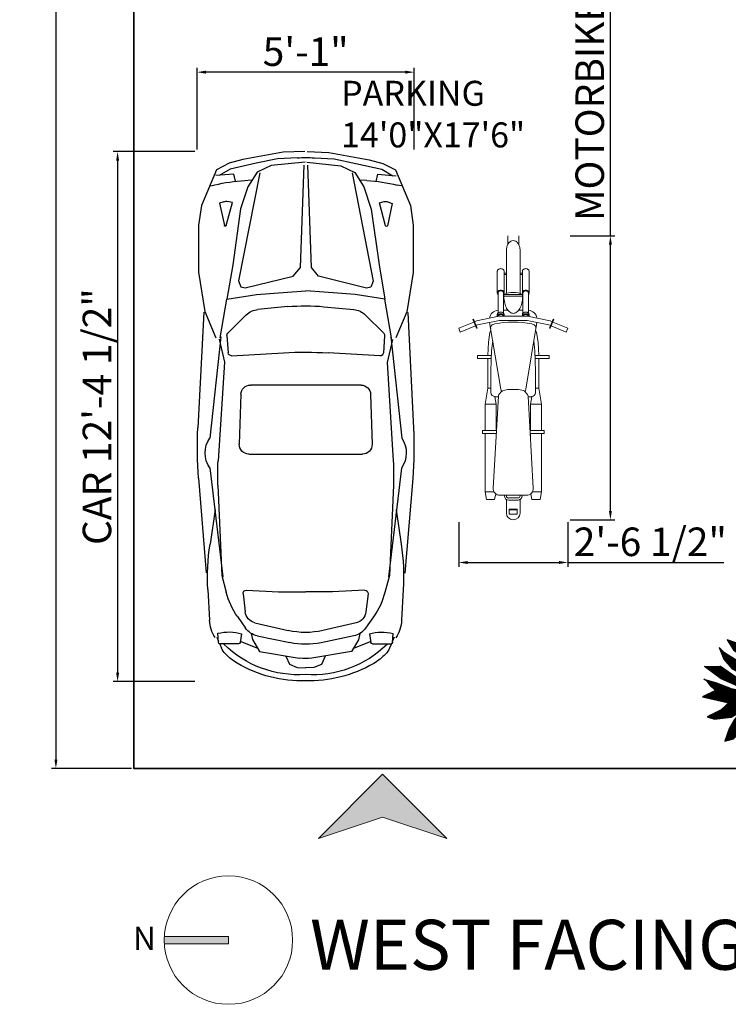
# Model space of a CAD drawing. Units: inches. Extents: x 1986 to 21484, y -1816 to 2016.
# Tile 1 of 85: x 2010 to 2209, y 1001 to 1277. Entities that reach past the tile are written whole.
import ezdxf

# ---------------------------------------------------------------- set-up
doc = ezdxf.new("R2010")
doc.units = ezdxf.units.IN
for name, color, linetype, lineweight in [('A-ANNO-DIMS', 2, 'Continuous', 18), ('A-ANNO-SYMB', 1, 'Continuous', 18), ('A-ANNO-TEXT', 7, 'Continuous', 18), ('A-AREA-IDEN', 3, 'Continuous', 18), ('A-EQPM', 9, 'Continuous', 18), ('C-PROP', 7, 'Continuous', 35), ('L-PLNT', 84, 'Continuous', 13), ('vfolhas', 114, 'Continuous', 5)]:
    doc.layers.add(name, color=color, linetype=linetype, lineweight=lineweight)
for name, color, linetype in [('L9012X$0', 2, 'Continuous'), ('vfolha', 72, 'Continuous'), ('vfolha2', 110, 'Continuous'), ('vfolhas2', 102, 'Continuous')]:
    doc.layers.add(name, color=color, linetype=linetype)
doc.styles.get("Standard").update_dxf_attribs({"font": 'arial.ttf'})
doc.dimstyles.new('ISO-25', dxfattribs={"dimtxt": 8, "dimasz": 2.5, "dimexe": 1.25, "dimexo": 0.625, "dimtad": 1, "dimdec": 1, "dimlunit": 3, "dimtxsty": 'Standard', "dimcen": 2.5, "dimadec": 0, "dimazin": 0, "dimtfac": 1, "dimtdec": 1, "dimtmove": 0, "dimatfit": 3, "dimfxl": 1, "dimarcsym": 0})
pattern_1 = [(45, (-2446.5133113, 50.986076), (-0.004419417382, 0.004419417382), [])]

# ---------------------------------------------------------------- blocks, each defined once
blk = doc.blocks.new('*D2')
at = {"layer": 'A-ANNO-DIMS', "color": 0, "lineweight": -2, "transparency": 16777216}
for p, q in [((2041.69, 1900.75), (2019.21, 1900.75)), ((2020.46, 1898.25), (2020.46, 1069.25)), ((2041.69, 1066.75), (2019.21, 1066.75))]:
    blk.add_line(p, q, dxfattribs=at)
at = {"layer": 'A-ANNO-DIMS', "color": 0, "transparency": 16777216}
for points in [[(2020.05, 1898.25), (2020.88, 1898.25), (2020.46, 1900.75)], [(2020.05, 1069.25), (2020.88, 1069.25), (2020.46, 1066.75)]]:
    blk.add_solid(points, dxfattribs=at)
at = {"layer": 'Defpoints', "color": 0, "transparency": 16777216}
for p in [(2042.31, 1900.75), (2020.46, 1066.75), (2042.31, 1066.75)]:
    blk.add_point(p, dxfattribs=at)
at = {"layer": 'A-ANNO-DIMS', "color": 0, "transparency": 16777216, "insert": (2015.75, 1483.75), "char_height": 8, "attachment_point": 5, "rotation": 90}
blk.add_mtext('69\'-6"', dxfattribs=at)
blk = doc.blocks.new('arbusto_PB_verde_grande')
at = {"layer": 'vfolha2'}
h = blk.add_hatch(dxfattribs=at)
h.set_pattern_fill('ANSI31', color=256, scale=0.05, style=0)
h.set_pattern_definition(pattern_1)
h.paths.add_polyline_path([(0.029, 0.357), (0, 0.09), (0.026, -0.039), (0.047, 0.062), (0.062, 0.097), (0.094, 0.266), (0.1, 0.435), (0.088, 0.613), (0.064, 0.723), (0.05, 0.685), (0.024, 0.513)])
h.paths.add_polyline_path([(0.301, 0.438), (0.142, 0.249), (0.267, 0.3)])
h.paths.add_polyline_path([(0.38, 0.228), (0.237, 0.152), (0.184, 0.094), (0.111, 0.044), (0.026, -0.039), (0.281, 0.047), (0.368, 0.078), (0.468, 0.112), (0.611, 0.194), (0.716, 0.278), (0.558, 0.259)])
h.paths.add_polyline_path([(0.561, -0.294), (0.728, -0.326), (0.59, -0.241), (0.43, -0.16), (0.026, -0.039), (0.149, -0.141), (0.188, -0.166), (0.415, -0.244)])
h.paths.add_polyline_path([(-0.274, -0.448), (-0.304, -0.726), (-0.239, -0.642), (-0.155, -0.457), (0.026, -0.039), (-0.163, -0.254)])
h.paths.add_polyline_path([(-0.52, -0.247), (-0.677, -0.326), (-0.596, -0.351), (-0.406, -0.329), (-0.21, -0.21), (0.026, -0.039), (-0.149, -0.066), (-0.315, -0.091), (-0.415, -0.15)])
h.paths.add_polyline_path([(-0.525, 0.25), (-0.709, 0.247), (-0.52, 0.109), (-0.33, 0.022), (-0.076, -0.013), (-0.042, -0.021), (-0.35, 0.131)])
h = blk.add_hatch(dxfattribs=at)
h.set_pattern_fill('ANSI31', color=256, scale=0.05, style=0)
h.set_pattern_definition(pattern_1)
h.paths.add_polyline_path([(-0.19, 0.297), (-0.086, 0.202), (-0.108, 0.25), (-0.132, 0.319), (-0.251, 0.485), (-0.45, 0.551), (-0.379, 0.438)])
h.paths.add_polyline_path([(0.079, -0.407), (0.082, -0.506), (0.173, -0.635), (0.184, -0.442), (0.149, -0.292), (0.026, -0.039), (0.035, -0.254)])
at = {"layer": 'vfolhas'}
h = blk.add_hatch(dxfattribs=at)
h.set_pattern_fill('ANSI31', color=256, scale=0.05, style=0)
h.set_pattern_definition(pattern_1)
h.paths.add_polyline_path([(-0.073, 0.507), (-0.181, 0.651), (-0.233, 0.673), (-0.207, 0.532), (-0.108, 0.25), (0.026, -0.039), (0, 0.09), (0.008, 0.162), (-0.049, 0.291)])
h.paths.add_polyline_path([(0.099, 0.419), (0.094, 0.266), (0.079, 0.188), (0.155, 0.369), (0.266, 0.551), (0.284, 0.635), (0.249, 0.688), (0.251, 0.635), (0.202, 0.544)])
h.paths.add_polyline_path([(0.123, 0.241), (0.047, 0.062), (0.026, -0.039), (0.111, 0.044), (0.184, 0.094), (0.275, 0.194), (0.322, 0.253), (0.441, 0.385), (0.476, 0.579), (0.418, 0.453), (0.289, 0.31)])
h.paths.add_polyline_path([(0.581, -0.038), (0.707, 0.015), (0.786, 0.047), (0.748, 0.065), (0.628, 0.084), (0.526, 0.09), (0.397, 0.044), (0.026, -0.039), (0.257, -0.032), (0.438, -0.035)])
h.paths.add_polyline_path([(0.52, -0.036), (0.438, -0.035), (0.257, -0.032), (0.026, -0.039), (0.18, -0.085), (0.538, -0.132), (0.695, -0.154), (0.786, -0.079), (0.704, -0.1)])
h.paths.add_polyline_path([(0.272, -0.219), (0.149, -0.141), (0.026, -0.039), (0.158, -0.31), (0.295, -0.426), (0.418, -0.492), (0.564, -0.567), (0.511, -0.485), (0.395, -0.341)])
h.paths.add_polyline_path([(-0.058, -0.476), (-0.023, -0.62), (0.047, -0.801), (0.085, -0.598), (0.079, -0.407), (0.035, -0.254), (0.026, -0.039), (-0.038, -0.26)])
h.paths.add_polyline_path([(-0.242, 0.141), (-0.111, 0.069), (0.026, -0.039), (-0.042, 0.109), (-0.21, 0.238), (-0.365, 0.331), (-0.479, 0.403), (-0.543, 0.463), (-0.49, 0.331), (-0.394, 0.222)])
h = blk.add_hatch(dxfattribs=at)
h.set_pattern_fill('ANSI31', color=256, scale=0.05, style=0)
h.set_pattern_definition(pattern_1)
h.paths.add_polyline_path([(-0.572, 0.062), (-0.715, 0.103), (-0.677, 0.081), (-0.628, 0.015), (-0.563, -0.041), (-0.265, -0.083), (-0.149, -0.066), (-0.102, -0.059), (-0.204, -0.047), (-0.403, -0.003)])
h.paths.add_polyline_path([(-0.563, -0.041), (-0.583, -0.024), (-0.73, -0.097), (-0.433, -0.168), (-0.415, -0.15), (-0.315, -0.091), (-0.265, -0.083)])
h.paths.add_polyline_path([(-0.277, -0.473), (-0.274, -0.448), (-0.163, -0.254), (0.026, -0.039), (-0.21, -0.21), (-0.267, -0.245), (-0.365, -0.357), (-0.429, -0.463), (-0.476, -0.604), (-0.379, -0.576)])
h = blk.add_hatch(dxfattribs=at)
h.set_pattern_fill('ANSI31', color=256, scale=0.05, style=0)
h.set_pattern_definition(pattern_1)
h.paths.add_polyline_path([(0.336, -0.623), (0.433, -0.673), (0.395, -0.595), (0.33, -0.445), (0.295, -0.426), (0.158, -0.31), (0.149, -0.292), (0.184, -0.442)])
at = {"layer": 'vfolha'}
for p, q in [((0.026, -0.039), (-0.149, -0.066)), ((0.026, -0.039), (-0.038, -0.26)), ((0.035, -0.254), (0.026, -0.039)), ((0.538, -0.132), (0.18, -0.085)), ((0.52, -0.036), (0.704, -0.1)), ((0.786, -0.079), (0.695, -0.154)), ((0.704, -0.1), (0.786, -0.079)), ((0.395, -0.341), (0.272, -0.219)), ((0.695, -0.154), (0.538, -0.132)), ((-0.267, -0.245), (-0.365, -0.357)), ((-0.038, -0.26), (-0.058, -0.476)), ((0.079, -0.407), (0.035, -0.254)), ((0.158, -0.31), (0.295, -0.426)), ((0.085, -0.598), (0.079, -0.407)), ((0.295, -0.426), (0.418, -0.492)), ((0.511, -0.485), (0.395, -0.341)), ((0.418, -0.492), (0.564, -0.567)), ((0.564, -0.567), (0.511, -0.485)), ((-0.023, -0.62), (0.047, -0.801)), ((0.047, -0.801), (0.085, -0.598))]:
    blk.add_line(p, q, dxfattribs=at)
at = {"layer": 'vfolha2'}
for p, q in [((0.024, 0.513), (0.05, 0.685)), ((0.05, 0.685), (0.064, 0.723)), ((0.064, 0.723), (0.088, 0.613)), ((0.088, 0.613), (0.1, 0.435)), ((-0.45, 0.551), (-0.379, 0.438)), ((-0.251, 0.485), (-0.45, 0.551)), ((-0.132, 0.319), (-0.251, 0.485)), ((0.029, 0.357), (0.024, 0.513)), ((-0.379, 0.438), (-0.19, 0.297)), ((0, 0.09), (0.029, 0.357)), ((0.1, 0.435), (0.094, 0.266)), ((0.143, 0.25), (0.301, 0.438)), ((0.301, 0.438), (0.266, 0.297)), ((-0.709, 0.247), (-0.525, 0.25)), ((-0.52, 0.109), (-0.709, 0.247)), ((-0.525, 0.25), (-0.35, 0.131)), ((-0.19, 0.297), (-0.082, 0.199)), ((0.237, 0.152), (0.38, 0.228)), ((0.38, 0.228), (0.558, 0.259)), ((0.558, 0.259), (0.716, 0.278)), ((0.716, 0.278), (0.611, 0.194)), ((-0.35, 0.131), (-0.042, -0.021)), ((0.611, 0.194), (0.468, 0.112)), ((-0.33, 0.022), (-0.52, 0.109)), ((-0.076, -0.013), (-0.33, 0.022)), ((0.026, -0.039), (0, 0.09)), ((0.281, 0.047), (0.026, -0.039)), ((0.368, 0.078), (0.281, 0.047)), ((-0.315, -0.091), (-0.415, -0.15)), ((-0.149, -0.066), (-0.315, -0.091)), ((-0.21, -0.21), (0.026, -0.039)), ((0.026, -0.039), (-0.163, -0.254)), ((-0.155, -0.457), (0.026, -0.039)), ((0.43, -0.16), (0.026, -0.039)), ((0.026, -0.039), (0.158, -0.31)), ((-0.415, -0.15), (-0.52, -0.247)), ((-0.406, -0.329), (-0.21, -0.21)), ((0.188, -0.166), (0.415, -0.244)), ((0.59, -0.241), (0.43, -0.16)), ((-0.52, -0.247), (-0.677, -0.326)), ((-0.677, -0.326), (-0.596, -0.351)), ((-0.596, -0.351), (-0.406, -0.329)), ((-0.163, -0.254), (-0.274, -0.448)), ((0.184, -0.442), (0.149, -0.292)), ((0.415, -0.244), (0.561, -0.294)), ((0.561, -0.294), (0.728, -0.326)), ((0.728, -0.326), (0.59, -0.241)), ((-0.274, -0.448), (-0.304, -0.726)), ((0.173, -0.635), (0.184, -0.442)), ((0.082, -0.506), (0.173, -0.635)), ((-0.304, -0.726), (-0.239, -0.642))]:
    blk.add_line(p, q, dxfattribs=at)
at = {"layer": 'vfolhas2'}
for p, q in [((0.251, 0.635), (0.249, 0.688)), ((0.249, 0.688), (0.284, 0.635)), ((-0.233, 0.673), (-0.207, 0.532)), ((-0.181, 0.651), (-0.233, 0.673)), ((-0.073, 0.507), (-0.181, 0.651)), ((0.202, 0.544), (0.251, 0.635)), ((0.284, 0.635), (0.266, 0.551)), ((0.418, 0.453), (0.476, 0.579)), ((0.476, 0.579), (0.441, 0.385)), ((-0.543, 0.463), (-0.49, 0.331)), ((-0.479, 0.403), (-0.543, 0.463)), ((-0.207, 0.532), (-0.108, 0.25)), ((-0.049, 0.291), (-0.073, 0.507)), ((0.099, 0.419), (0.202, 0.544)), ((0.266, 0.551), (0.155, 0.369)), ((0.289, 0.31), (0.418, 0.453)), ((-0.365, 0.331), (-0.479, 0.403)), ((0.155, 0.369), (0.078, 0.186)), ((0.441, 0.385), (0.322, 0.253)), ((-0.49, 0.331), (-0.394, 0.222)), ((-0.21, 0.238), (-0.365, 0.331)), ((-0.042, 0.109), (-0.21, 0.238)), ((-0.108, 0.25), (0.026, -0.039)), ((0.008, 0.162), (-0.049, 0.291)), ((0.047, 0.062), (0.123, 0.241)), ((0.094, 0.266), (0.062, 0.097)), ((0.123, 0.241), (0.289, 0.31)), ((0.322, 0.253), (0.275, 0.194)), ((-0.394, 0.222), (-0.242, 0.141)), ((-0.242, 0.141), (-0.111, 0.069)), ((0.275, 0.194), (0.184, 0.094)), ((0.468, 0.112), (0.368, 0.078)), ((-0.677, 0.081), (-0.715, 0.103)), ((-0.715, 0.103), (-0.572, 0.062)), ((-0.628, 0.015), (-0.677, 0.081)), ((-0.563, -0.041), (-0.628, 0.015)), ((-0.572, 0.062), (-0.403, -0.003)), ((-0.111, 0.069), (0.026, -0.039)), ((0.026, -0.039), (0.047, 0.062)), ((0.026, -0.039), (0.397, 0.044)), ((0.111, 0.044), (0.026, -0.039)), ((0.184, 0.094), (0.111, 0.044)), ((0.397, 0.044), (0.526, 0.09)), ((0.526, 0.09), (0.628, 0.084)), ((0.707, 0.015), (0.581, -0.038)), ((0.628, 0.084), (0.748, 0.065)), ((0.786, 0.047), (0.707, 0.015)), ((0.748, 0.065), (0.786, 0.047)), ((-0.583, -0.024), (-0.73, -0.097)), ((-0.73, -0.097), (-0.433, -0.168)), ((-0.265, -0.083), (-0.563, -0.041)), ((-0.403, -0.003), (-0.204, -0.047)), ((-0.204, -0.047), (-0.098, -0.059)), ((0.026, -0.039), (-0.076, -0.013)), ((0.257, -0.032), (0.026, -0.039)), ((0.149, -0.141), (0.026, -0.039)), ((0.438, -0.035), (0.257, -0.032)), ((0.581, -0.038), (0.438, -0.035)), ((0.272, -0.219), (0.149, -0.141)), ((-0.365, -0.357), (-0.429, -0.463)), ((0.184, -0.442), (0.336, -0.623)), ((0.395, -0.595), (0.329, -0.442)), ((-0.429, -0.463), (-0.476, -0.604)), ((-0.379, -0.576), (-0.277, -0.473)), ((-0.239, -0.642), (-0.155, -0.457)), ((-0.058, -0.476), (-0.023, -0.62)), ((-0.476, -0.604), (-0.379, -0.576)), ((0.336, -0.623), (0.433, -0.673)), ((0.433, -0.673), (0.395, -0.595))]:
    blk.add_line(p, q, dxfattribs=at)
blk = doc.blocks.new('A1099DC')
at = {"color": 0, "linetype": 'ByBlock'}
for p, q in [((1279.298465, 804.448389), (2201.430588, 851.890505)), ((2602.736326, 846.078152), (3356.693814, 785.353187)), ((179.200345, 564.515703), (190.951238, 709.631982)), ((272.228253, 749.073842), (265.114727, 718.465169)), ((1475.52921, 670.226262), (2282.402739, 758.004075)), ((2519.280414, 756.817792), (3387.476361, 653.818028)), ((2851.341839, 715.213377), (3126.60716, 755.701993)), ((3488.458929, 772.663345), (3732.658862, 759.86454)), ((139.051458, 595.027331), (190.951238, 683.213377)), ((398.733388, 644.315148), (411.280494, 678.748261)), ((411.280494, 678.748261), (588.616917, 641.417897)), ((1482.852352, 674.283145), (1175.286956, 622.180789)), ((1494.603245, 682.841284), (1678.210958, 641.166865)), ((1678.210958, 641.166865), (2462.684993, 690.847736)), ((2656.476214, 692.831247), (3376.704709, 662.004075)), ((3376.704709, 662.004075), (3510.708679, 626.736433)), ((3909.27561, 688.812956), (3837.725727, 693.401722)), ((3867.794139, 700.329656), (3900.059395, 686.767505)), ((3921.162781, 527.618662), (3921.162781, 676.138994)), ((3925.383812, 676.122818), (3955.306409, 663.545364)), ((92.537504, 388.14361), (139.051458, 595.027331)), ((236.043912, 551.980927), (179.200345, 564.515703)), ((405.405047, 577.538958), (396.874865, 615.894428)), ((589.014326, 626.599587), (405.405047, 577.538958)), ((1300.814287, 466.658131), (1445.712032, 613.104998)), ((1465.665584, 620.56924), (1602.893878, 610.287296)), ((1626.354615, 583.507504), (1602.652901, 169.222264)), ((229.117398, 477.634662), (225.714299, 427.957563)), ((1933.148906, 509.557888), (2330.980062, 522.200075)), ((3522.252709, 492.345257), (3666.066199, 475.644444)), ((3704.596898, 536.993674), (3795.675135, 473.385795)), ((3841.786866, 503.451367), (3910.58243, 515.096797)), ((3901.001848, 514.780764), (3957.150905, 375.772812)), ((1860.238743, -448.635916), (1859.369151, 433.397797)), ((2409.60024, 445.938054), (2410.49349, -460.09121)), ((3493.960271, 465.734554), (3507.923021, 209.166865)), ((3753.293176, 397.789551), (3815.226005, 132.124765)), ((3839.396146, 426.841284), (3888.358202, 417.538958)), ((3888.358202, 417.538958), (3983.199613, 359.957848)), ((57.774444, 216.608726), (92.537504, 388.14361)), ((1235.045743, 136.116317), (1257.419842, 373.755108)), ((3857.610793, 379.525702), (3912.067615, 118.157673)), ((3983.199613, 359.957848), (4035.448301, 43.94997)), ((49.168662, 58.00681), (57.774444, 216.608726)), ((3507.923021, 209.166865), (3507.64153, -4.333678)), ((4019.086894, 150.376168), (4084.69605, 122.469191)), ((4084.69605, 122.469191), (4109.177079, 60.329656)), ((4109.177079, 60.329656), (4113.094043, -5.158716)), ((49.301278, -76.507426), (58.219773, -235.092064)), ((3508.347273, -221.154823), (3507.644805, -7.65525)), ((3983.920268, -371.008369), (4035.545755, -54.898082)), ((4084.948231, -133.320044), (4109.306686, -71.132359)), ((4109.306686, -71.132359), (4113.094514, -5.636391)), ((1235.330373, -152.586046), (1258.173002, -390.180259)), ((3754.088875, -409.293325), (3815.497749, -143.506937)), ((3858.370276, -390.823819), (3912.311631, -129.348921)), ((4019.394229, -161.356334), (4084.948231, -133.320044)), ((58.219773, -235.092064), (93.320996, -406.558069)), ((1627.520644, -599.204785), (1603.002095, -184.967086)), ((3494.890446, -477.749545), (3508.347273, -221.154823)), ((3889.19258, -428.776374), (3983.920268, -371.008369)), ((3902.027941, -525.993061), (3957.902795, -386.874665)), ((93.320996, -406.558069), (140.24279, -613.349673)), ((230.077082, -495.779641), (226.576036, -446.109349)), ((3840.248961, -438.175225), (3889.19258, -428.776374)), ((1301.750547, -482.997536), (1446.936772, -629.158411)), ((1934.168526, -524.650381), (2332.023837, -536.508105)), ((3523.2353, -504.304409), (3667.01558, -487.320059)), ((3705.667171, -548.593196), (3796.61981, -484.805853)), ((3842.790735, -514.780444), (3911.609128, -526.290202)), ((3922.214148, -538.79118), (3922.506998, -687.311224)), ((140.24279, -613.349673), (192.316354, -701.433212)), ((237.150178, -570.112104), (180.331436, -582.758939)), ((180.331436, -582.758939), (192.368445, -727.851766)), ((406.561378, -595.336142), (398.106841, -633.708356)), ((590.267037, -644.034637), (406.561378, -595.336142)), ((1466.905004, -636.583294), (1604.112757, -626.030785)), ((400.0214, -662.125356), (412.636377, -696.533662)), ((412.636377, -696.533662), (589.898847, -658.853701)), ((1484.19765, -690.263206), (1176.530118, -638.767405)), ((1476.866524, -686.22077), (2283.911563, -772.40743)), ((1495.965396, -698.798158), (1679.490579, -656.761786)), ((1679.490579, -656.761786), (2464.061049, -704.895745)), ((2520.786439, -770.754078), (3388.777604, -666.042617)), ((2657.855804, -706.497136), (3378.022114, -674.249887)), ((3378.022114, -674.249887), (3511.956283, -638.718087)), ((3910.644841, -700.0086), (3839.104145, -704.738438)), ((3869.186159, -711.60707), (3901.424611, -697.981326)), ((3926.727989, -687.286725), (3956.625729, -674.650294)), ((273.723073, -767.133288), (266.549207, -736.538701)), ((2852.765183, -728.494989), (3128.109803, -768.440762)), ((3489.994314, -784.688586), (3734.168535, -771.408296)), ((1280.900818, -820.829563), (2203.124693, -866.453338)), ((2604.418191, -859.849707), (3358.254477, -797.638217))]:
    blk.add_line(p, q, dxfattribs=at)
for points in [[(-0.000783, 0.794772), (5.385043, 172.701749), (63.649891, 493.818028), (92.537504, 603.957563), (144.437284, 705.166865), (428.417214, 824.236633), (585.095796, 846.190121), (961.406447, 846.190121), (1274.27399, 797.818028), (1482.852352, 709.631982)], [(83.345007, -3.206171), (111.32237, 268.957533), (164.563706, 379.583828), (279.999271, 453.709838), (456.549665, 511.628518), (901.254996, 574.918954), (1175.286956, 622.180789), (1137.52997, 385.548359), (1118.345181, 137.317882), (1109.829198, -8.358455)], [(168.178729, 359.003083), (1030.214866, 528.397865), (1077.798844, 510.531569), (1086.170082, 475.285426), (992.832238, 91.960378), (924.218938, 35.478085), (108.447994, 6.034416)], [(0.019119, -19.392451), (5.743899, -191.288474), (64.641806, -512.289243), (93.746535, -622.371603), (145.845778, -723.478374), (430.059935, -841.987962), (586.7815, -863.632471), (963.091723, -863.198028), (1275.863278, -814.209121), (1484.26735, -725.611974)], [(83.356858, -15.227176), (111.870816, -287.335185), (165.330179, -397.856284), (280.911681, -471.754535), (457.575935, -529.324983), (902.4055, -592.045995), (1176.530118, -638.767405), (1138.306616, -402.209884), (1118.632407, -154.017717), (1109.829198, -8.358455)], [(168.904615, -377.268451), (1031.273389, -545.270714), (1078.822046, -527.310627), (1087.123771, -492.048047), (993.030273, -108.907787), (924.305735, -52.560894), (108.478017, -24.418246)]]:
    blk.add_lwpolyline(points, dxfattribs=at)
for centre, radius, start, end in [((2358.037832, -2192.08357), 3048, 85.395244, 92.945173), ((2399.99649, 588.663508), 206.166238, 54.649181, 124.776949), ((1749.553982, 373.478072), 1524, 166.916578, 176.08111), ((3392.740754, -1053.630025), 1828.8, 86.999806, 98.367602), ((3718.678317, 475.802507), 284.405862, 57.329946, 87.182375), ((446.46332, 626.922805), 50.8, 159.97873, 192.538409), ((587.047263, 633.961317), 7.62, 284.960009, 78.112462), ((2578.271641, -1134.295865), 1828.8, 87.549126, 93.623712), ((4191.049821, 605.937201), 363.988953, 166.096081, 196.353514), ((3908.462781, 676.138994), 12.7, 0, 86.330429), ((3320.85101, 50.338397), 847.430844, 356.245089, 44.519453), ((3896.252417, 523.051998), 152.4, 46.38363, 67.20138), ((3700.933354, 318.064082), 435.542335, 30.457681, 46.38363), ((1463.767788, 595.240237), 25.4, 85.715073, 135.304647), ((1600.996082, 584.958293), 25.4, 356.725615, 85.715073), ((3355.555414, 37.211519), 609.6, 55.070043, 75.255062), ((1935.569151, 433.396333), 76.2, 91.82012, 179.9989), ((2333.400307, 446.03852), 76.2, 359.924458, 91.82012), ((3519.322741, 467.114813), 25.4, 83.37601, 183.115039), ((3654.346327, 374.722669), 101.6, 13.122645, 83.37601), ((3708.414764, 348.440256), 152.4, 11.769371, 55.070043), ((3908.462781, 527.618662), 12.7, 279.607718, 0), ((3204.184594, 25.950693), 1011.814461, 358.069446, 30.457681), ((1409.148822, 359.469565), 152.4, 135.304647, 174.62136), ((4645.676894, -4.872483), 3048, 176.725615, 183.38736), ((2752.335538, -6.739118), 1524, 174.62136, 185.491615), ((3221.54491, -6.276527), 609.6, 346.99033, 13.122645), ((3315.283499, -6.18411), 609.6, 348.343604, 11.769371), ((1266.577845, -8.050136), 1219.2, 176.894161, 183.218814), ((3734.73098, -5.770579), 304.8, 350.724636, 9.388339), ((3320.962449, -62.69553), 847.430844, 315.593523, 3.867886), ((3204.248172, -38.537915), 1011.814461, 329.655294, 2.043529), ((1409.873518, -375.595566), 152.4, 185.491615, 224.808328), ((3709.113243, -360.032616), 152.4, 305.042932, 348.343604), ((1936.438592, -448.484202), 76.2, 180.114076, 268.292856), ((2334.293902, -460.341926), 76.2, 268.292856, 0.188517), ((3655.096735, -386.42159), 101.6, 276.736965, 346.99033), ((1750.305335, -388.625277), 1524, 184.031865, 193.196397), ((3520.255588, -479.079792), 25.4, 176.997936, 276.736965), ((3355.640902, -49.500248), 609.6, 284.857913, 305.042932), ((4192.255091, -616.577407), 363.988953, 163.759461, 194.016894), ((3909.514173, -538.816222), 12.7, 0.112975, 80.505257), ((1602.165021, -600.705574), 25.4, 274.397903, 3.38736), ((3701.571953, -329.671253), 435.542335, 313.729345, 329.655294), ((447.716945, -644.638934), 50.8, 167.574566, 200.134245), ((588.314493, -651.400231), 7.62, 282.000513, 75.152966), ((1464.957267, -611.258083), 25.4, 224.808328, 274.397903), ((2576.048678, 1120.472221), 1828.8, 266.489263, 272.563849), ((3909.807023, -687.336265), 12.7, 273.782546, 0.112975), ((3897.294828, -534.273643), 152.4, 292.911596, 313.729345), ((2401.171182, -602.835323), 206.166238, 235.336026, 305.463794), ((3390.675263, 1041.412497), 1828.8, 261.745373, 273.113169), ((3719.627907, -487.374382), 284.405862, 272.930601, 302.78303), ((2353.729565, 2177.823616), 3048, 267.167802, 274.717731)]:
    blk.add_arc(centre, radius, start, end, dxfattribs=at)
blk = doc.blocks.new('VI')
at = {"layer": 'L9012X$0'}
blk.add_blockref('A1099DC', (0, 0), dxfattribs=at)
blk = doc.blocks.new('BIKE')
for p, q in [((34846.04, 15170.34), (34846.04, 15168.87)), ((34847.86, 15170.34), (34847.86, 15168.87)), ((34845.81, 15167.86), (34845.81, 15160.7)), ((34845.81, 15167.86), (34845.81, 15160.7)), ((34848.09, 15167.86), (34848.09, 15160.7)), ((34844.29, 15164.4), (34844.29, 15160.81)), ((34845.43, 15164.4), (34845.43, 15160.81)), ((34845.43, 15164.1), (34845.81, 15164.1)), ((34845.43, 15163.85), (34845.81, 15163.85)), ((34848.47, 15164.1), (34848.09, 15164.1)), ((34848.47, 15163.85), (34848.09, 15163.85)), ((34848.47, 15164.4), (34848.47, 15160.81)), ((34849.61, 15164.4), (34849.61, 15160.81)), ((34844.41, 15160.81), (34844.41, 15157.43)), ((34845.32, 15160.81), (34845.32, 15157.43)), ((34848.58, 15160.81), (34848.58, 15157.43)), ((34849.5, 15160.81), (34849.5, 15157.43)), ((34848.51, 15160.53), (34845.39, 15160.53)), ((34845.39, 15160.23), (34845.39, 15160.53)), ((34845.39, 15160.23), (34845.39, 15160.53)), ((34848.51, 15160.23), (34845.39, 15160.23)), ((34848.51, 15160.23), (34848.51, 15160.53)), ((34845.32, 15157.92), (34846.04, 15157.92)), ((34848.58, 15157.92), (34847.87, 15157.92)), ((34837.84, 15154.89), (34840.37, 15155.93)), ((34840.19, 15156.35), (34840.3, 15156.39)), ((34840.19, 15156.35), (34840.8, 15154.88)), ((34840.3, 15156.39), (34840.9, 15154.92)), ((34840.47, 15155.97), (34840.8, 15156.11)), ((34840.8, 15156.11), (34844.56, 15156.88)), ((34841, 15155.45), (34844.63, 15156.2)), ((34844.86, 15144.72), (34843.01, 15155.87)), ((34844.29, 15156.87), (34844.29, 15157.17)), ((34844.41, 15156.87), (34844.41, 15156.85)), ((34844.56, 15156.88), (34846.95, 15156.88)), ((34844.63, 15156.2), (34846.95, 15156.2)), ((34845.43, 15156.87), (34845.43, 15157.17)), ((34849.34, 15156.88), (34846.95, 15156.88)), ((34849.27, 15156.2), (34846.95, 15156.2)), ((34848.47, 15156.87), (34848.47, 15157.17)), ((34849.05, 15144.72), (34850.89, 15155.87)), ((34852.9, 15155.45), (34849.27, 15156.2)), ((34853.1, 15156.11), (34849.34, 15156.88)), ((34849.5, 15156.87), (34849.5, 15156.85)), ((34849.61, 15156.87), (34849.61, 15157.17)), ((34853.6, 15156.39), (34853, 15154.92)), ((34853.71, 15156.35), (34853.1, 15154.88)), ((34853.43, 15155.97), (34853.1, 15156.11)), ((34856.07, 15154.89), (34853.54, 15155.93)), ((34853.71, 15156.35), (34853.6, 15156.39)), ((34837.84, 15154.89), (34838.1, 15154.26)), ((34838.1, 15154.26), (34840.63, 15155.3)), ((34840.73, 15155.34), (34841, 15155.45)), ((34840.8, 15154.88), (34840.9, 15154.92)), ((34842.8, 15152.59), (34843.06, 15154.2)), ((34843.06, 15154.2), (34843.22, 15154.58)), ((34850.84, 15154.2), (34850.68, 15154.58)), ((34851.1, 15152.59), (34850.84, 15154.2)), ((34853.17, 15155.34), (34852.9, 15155.45)), ((34853.1, 15154.88), (34853, 15154.92)), ((34855.81, 15154.26), (34853.28, 15155.3)), ((34856.07, 15154.89), (34855.81, 15154.26)), ((34842.7, 15150.31), (34842.8, 15152.59)), ((34843.33, 15151.09), (34843.52, 15152.8)), ((34850.57, 15151.09), (34850.38, 15152.8)), ((34851.2, 15150.31), (34851.1, 15152.59)), ((34843.23, 15147.75), (34843.33, 15151.09)), ((34850.67, 15147.75), (34850.57, 15151.09)), ((34840.97, 15150.31), (34843.3, 15150.31)), ((34840.97, 15149.81), (34840.97, 15150.31)), ((34843.29, 15149.81), (34840.97, 15149.81)), ((34842.7, 15144.87), (34842.7, 15149.81)), ((34852.93, 15150.31), (34850.6, 15150.31)), ((34850.61, 15149.81), (34852.93, 15149.81)), ((34851.2, 15144.87), (34851.2, 15149.81)), ((34852.93, 15149.81), (34852.93, 15150.31)), ((34843.23, 15144.15), (34843.23, 15147.75)), ((34850.67, 15144.15), (34850.67, 15147.75)), ((34842.7, 15144.87), (34842.25, 15142.19)), ((34842.7, 15144.87), (34843.23, 15144.87)), ((34847.85, 15144.64), (34846.06, 15144.64)), ((34851.2, 15144.87), (34850.67, 15144.87)), ((34851.2, 15144.87), (34851.65, 15142.19)), ((34844.46, 15143.56), (34843.6, 15128.2)), ((34843.85, 15143.46), (34844.07, 15142.19)), ((34843.91, 15143.46), (34844.46, 15143.46)), ((34849.44, 15143.56), (34850.3, 15128.2)), ((34849.99, 15143.46), (34849.44, 15143.46)), ((34850.05, 15143.46), (34849.83, 15142.19)), ((34842.25, 15142.19), (34844.07, 15142.19)), ((34842.25, 15137.82), (34842.25, 15142.19)), ((34844.07, 15137.82), (34844.07, 15142.19)), ((34851.65, 15142.19), (34849.83, 15142.19)), ((34849.83, 15137.82), (34849.83, 15142.19)), ((34851.65, 15137.82), (34851.65, 15142.19)), ((34841.79, 15137.82), (34844.14, 15137.82)), ((34841.79, 15137.33), (34841.79, 15137.82)), ((34852.11, 15137.82), (34849.76, 15137.82)), ((34852.11, 15137.33), (34852.11, 15137.82)), ((34844.11, 15137.33), (34841.79, 15137.33)), ((34842.25, 15127.57), (34842.25, 15137.33)), ((34844.07, 15136.55), (34844.07, 15137.33)), ((34849.79, 15137.33), (34852.11, 15137.33)), ((34849.83, 15136.55), (34849.83, 15137.33)), ((34851.65, 15127.57), (34851.65, 15137.33)), ((34842.25, 15127.57), (34843.75, 15127.57)), ((34842.25, 15127.57), (34842.48, 15126.27)), ((34842.48, 15126.27), (34843.84, 15126.27)), ((34844.02, 15127.25), (34843.84, 15126.27)), ((34849.16, 15126.99), (34844.74, 15126.99)), ((34845.47, 15126.99), (34845.47, 15126.88)), ((34845.81, 15126.99), (34845.81, 15126.88)), ((34845.81, 15126.29), (34845.81, 15124.03)), ((34847.75, 15126.54), (34846.15, 15126.54)), ((34847.75, 15126.2), (34846.15, 15126.2)), ((34848.09, 15126.99), (34848.09, 15126.88)), ((34848.09, 15126.29), (34848.09, 15124.03)), ((34848.43, 15126.99), (34848.43, 15126.88)), ((34849.89, 15127.25), (34850.06, 15126.27)), ((34851.43, 15126.27), (34850.06, 15126.27)), ((34851.65, 15127.57), (34850.15, 15127.57)), ((34851.65, 15127.57), (34851.43, 15126.27)), ((34846.29, 15123.82), (34846.29, 15124.66)), ((34846.29, 15124.66), (34847.61, 15124.66)), ((34846.29, 15124.55), (34847.61, 15124.55)), ((34847.61, 15124.66), (34847.61, 15123.82)), ((34847.61, 15123.82), (34846.29, 15123.82))]:
    blk.add_line(p, q)
for points in [[(34845.81, 15167.86, -0.068977), (34845.9, 15168.53, -0.081012), (34846.15, 15169.05, -0.107014), (34846.54, 15169.42, -0.137239), (34846.95, 15169.53, -0.137239), (34847.36, 15169.42, -0.107014), (34847.76, 15169.05, -0.081012), (34848, 15168.53, -0.068977), (34848.09, 15167.86, -0.068977)], [(34845.43, 15164.4, 0.125099), (34845.39, 15164.56, 0.105827), (34845.27, 15164.71, 0.086577), (34845.09, 15164.8, 0.0766), (34844.86, 15164.84, 0.0766), (34844.64, 15164.8, 0.086577), (34844.46, 15164.71, 0.105827), (34844.33, 15164.56, 0.125099), (34844.29, 15164.4, 0.125099)], [(34848.47, 15164.4, -0.125099), (34848.51, 15164.56, -0.105827), (34848.64, 15164.71, -0.086577), (34848.82, 15164.8, -0.0766), (34849.04, 15164.84, -0.0766), (34849.26, 15164.8, -0.086577), (34849.44, 15164.71, -0.105827), (34849.57, 15164.56, -0.125099), (34849.61, 15164.4, -0.125099)], [(34845.32, 15160.55, 0.067261), (34845.39, 15160.65, 0.125099), (34845.43, 15160.81, 0.125099), (34845.39, 15160.97, 0.105827), (34845.27, 15161.12, 0.086577), (34845.09, 15161.21, 0.0766), (34844.86, 15161.25, 0.0766), (34844.64, 15161.21, 0.086577), (34844.46, 15161.12, 0.105827), (34844.33, 15160.97, 0.125099), (34844.29, 15160.81, 0.125099)], [(34844.29, 15160.81, 0.125099), (34844.33, 15160.65, 0.067261), (34844.41, 15160.55, 0.086577)], [(34845.32, 15160.81, 0.125099), (34845.29, 15160.92, 0.105827), (34845.2, 15161.03, 0.086577), (34845.05, 15161.1, 0.0766), (34844.86, 15161.13, 0.0766), (34844.67, 15161.1, 0.086577), (34844.53, 15161.03, 0.105827), (34844.43, 15160.92, 0.125099), (34844.41, 15160.81, 0.125099)], [(34848.58, 15160.55, -0.067261), (34848.51, 15160.65, -0.125099), (34848.47, 15160.81, -0.125099), (34848.51, 15160.97, -0.105827), (34848.64, 15161.12, -0.086577), (34848.82, 15161.21, -0.0766), (34849.04, 15161.25, -0.0766), (34849.26, 15161.21, -0.086577), (34849.44, 15161.12, -0.105827), (34849.57, 15160.97, -0.125099), (34849.61, 15160.81, -0.125099)], [(34848.58, 15160.81, -0.125099), (34848.61, 15160.92, -0.105827), (34848.71, 15161.03, -0.086577), (34848.85, 15161.1, -0.0766), (34849.04, 15161.13, -0.0766), (34849.23, 15161.1, -0.086577), (34849.37, 15161.03, -0.105827), (34849.47, 15160.92, -0.125099), (34849.5, 15160.81, -0.125099)], [(34849.61, 15160.81, -0.125099), (34849.57, 15160.65, -0.067261), (34849.5, 15160.55, -0.086577)], [(34846.95, 15157.37, -0.163989), (34846.41, 15157.55, -0.105862), (34845.85, 15158.21, -0.069323), (34845.52, 15159.08, -0.055531), (34845.39, 15160.23, -0.055531)], [(34848.51, 15160.23, -0.055531), (34848.38, 15159.08, -0.069323), (34848.06, 15158.21, -0.105862), (34847.49, 15157.55, -0.163989), (34846.95, 15157.37, -0.163989)], [(34845.43, 15157.17, 0.125099), (34845.39, 15157.33, 0.105827), (34845.27, 15157.48, 0.086577), (34845.09, 15157.57, 0.0766), (34844.86, 15157.6, 0.0766), (34844.64, 15157.57, 0.086577), (34844.46, 15157.48, 0.105827), (34844.33, 15157.33, 0.125099), (34844.29, 15157.17, 0.125099)], [(34845.43, 15156.88, 0.117252), (34845.39, 15157.03, 0.105827), (34845.27, 15157.18, 0.086577), (34845.09, 15157.27, 0.0766), (34844.86, 15157.31, 0.0766), (34844.64, 15157.27, 0.086577), (34844.46, 15157.18, 0.105827), (34844.33, 15157.03, 0.125099), (34844.29, 15156.87, 0.125099)], [(34848.47, 15157.17, -0.125099), (34848.51, 15157.33, -0.105827), (34848.64, 15157.48, -0.086577), (34848.82, 15157.57, -0.0766), (34849.04, 15157.6, -0.0766), (34849.26, 15157.57, -0.086577), (34849.44, 15157.48, -0.105827), (34849.57, 15157.33, -0.125099), (34849.61, 15157.17, -0.125099)], [(34848.47, 15156.88, -0.117252), (34848.51, 15157.03, -0.105827), (34848.64, 15157.18, -0.086577), (34848.82, 15157.27, -0.0766), (34849.04, 15157.31, -0.0766), (34849.26, 15157.27, -0.086577), (34849.44, 15157.18, -0.105827), (34849.57, 15157.03, -0.125099), (34849.61, 15156.87, -0.125099)], [(34844.29, 15156.87, 0.032819), (34844.3, 15156.83, 0.067261)], [(34845.32, 15156.88, 0.113202), (34845.29, 15156.98, 0.105827), (34845.2, 15157.09, 0.086577), (34845.05, 15157.16, 0.0766), (34844.86, 15157.19, 0.0766), (34844.67, 15157.16, 0.086577), (34844.53, 15157.09, 0.105827), (34844.43, 15156.98, 0.125099), (34844.41, 15156.87, 0.125099)], [(34848.58, 15156.88, -0.113202), (34848.61, 15156.98, -0.105827), (34848.71, 15157.09, -0.086577), (34848.85, 15157.16, -0.0766), (34849.04, 15157.19, -0.0766), (34849.23, 15157.16, -0.086577), (34849.37, 15157.09, -0.105827), (34849.47, 15156.98, -0.125099), (34849.5, 15156.87, -0.125099)], [(34849.61, 15156.87, -0.032819), (34849.61, 15156.83, -0.067261)]]:
    blk.add_lwpolyline(points, format="xyb")
for centre, radius, start, end in [((34846.95, 15157.24), 3.64, 64.5882, 115.4118), ((34844.55, 15156.32), 1.59, 95.2207, 171.678), ((34849.35, 15156.32), 1.59, 8.322, 84.7793), ((34846.95, 15140.12), 15.79, 78.7129, 101.2871), ((34843.86, 15154.92), 0.684, 90, 189.3898), ((34850.04, 15154.92), 0.684, 350.6102, 90), ((34843.91, 15144.15), 0.684, 180, 270), ((34846, 15143), 1.64, 88.1125, 159.9264), ((34845.53, 15144.83), 0.684, 189.3898, 226.4877), ((34847.9, 15143), 1.64, 20.0736, 91.8875), ((34848.37, 15144.83), 0.684, 313.5123, 350.6102), ((34849.99, 15144.15), 0.684, 270, 0), ((34844.74, 15128.13), 1.14, 176.7865, 270), ((34849.16, 15128.13), 1.14, 270, 3.2135), ((34846.15, 15126.88), 0.684, 180, 270), ((34846.15, 15126.88), 0.342, 180, 270), ((34847.75, 15126.88), 0.684, 270, 0), ((34847.75, 15126.88), 0.342, 270, 0), ((34846.95, 15124.03), 1.14, 180, 0)]:
    blk.add_arc(centre, radius, start, end)
blk = doc.blocks.new('*D117')
at = {"layer": 'A-ANNO-DIMS', "color": 0, "lineweight": -2, "transparency": 16777216}
for p, q in [((2059.43, 1239.68), (2036.52, 1239.68)), ((2037.77, 1237.18), (2037.77, 1093.6)), ((2059.43, 1091.1), (2036.52, 1091.1))]:
    blk.add_line(p, q, dxfattribs=at)
at = {"layer": 'A-ANNO-DIMS', "color": 0, "transparency": 16777216}
for points in [[(2037.35, 1237.18), (2038.19, 1237.18), (2037.77, 1239.68)], [(2037.35, 1093.6), (2038.19, 1093.6), (2037.77, 1091.1)]]:
    blk.add_solid(points, dxfattribs=at)
at = {"layer": 'Defpoints', "color": 0, "transparency": 16777216}
for p in [(2060.06, 1239.68), (2037.77, 1091.1), (2060.06, 1091.1)]:
    blk.add_point(p, dxfattribs=at)
at = {"layer": 'A-ANNO-DIMS', "color": 0, "transparency": 16777216, "insert": (2033.01, 1165.39), "char_height": 8, "attachment_point": 5, "rotation": 90}
blk.add_mtext('CAR 12\'-4 1/2"', dxfattribs=at)
blk = doc.blocks.new('*D118')
at = {"layer": 'A-ANNO-DIMS', "color": 0, "lineweight": -2, "transparency": 16777216}
for p, q in [((2060.06, 1240.3), (2060.06, 1263.21)), ((2118.5, 1261.96), (2062.56, 1261.96)), ((2121, 1240.3), (2121, 1263.21))]:
    blk.add_line(p, q, dxfattribs=at)
at = {"layer": 'A-ANNO-DIMS', "color": 0, "transparency": 16777216}
for points in [[(2062.56, 1262.38), (2062.56, 1261.55), (2060.06, 1261.96)], [(2118.5, 1262.38), (2118.5, 1261.55), (2121, 1261.96)]]:
    blk.add_solid(points, dxfattribs=at)
at = {"layer": 'Defpoints', "color": 0, "transparency": 16777216}
for p in [(2060.06, 1261.96), (2060.06, 1239.68), (2121, 1239.68)]:
    blk.add_point(p, dxfattribs=at)
at = {"layer": 'A-ANNO-DIMS', "color": 0, "transparency": 16777216, "insert": (2090.53, 1266.67), "char_height": 8, "attachment_point": 5}
blk.add_mtext('5\'-1"', dxfattribs=at)
blk = doc.blocks.new('*D125')
at = {"layer": 'A-ANNO-DIMS', "color": 0, "lineweight": -2, "transparency": 16777216}
for p, q in [((2176.01, 1216.11), (2176.01, 1329.57)), ((2164.68, 1216.11), (2177.26, 1216.11)), ((2176.01, 1138.94), (2176.01, 1213.61)), ((2164.68, 1136.44), (2177.26, 1136.44))]:
    blk.add_line(p, q, dxfattribs=at)
at = {"layer": 'A-ANNO-DIMS', "color": 0, "transparency": 16777216}
for points in [[(2175.59, 1213.61), (2176.42, 1213.61), (2176.01, 1216.11)], [(2175.59, 1138.94), (2176.42, 1138.94), (2176.01, 1136.44)]]:
    blk.add_solid(points, dxfattribs=at)
at = {"layer": 'Defpoints', "color": 0, "transparency": 16777216}
for p in [(2164.06, 1216.11), (2176.01, 1216.11), (2164.06, 1136.44)]:
    blk.add_point(p, dxfattribs=at)
at = {"layer": 'A-ANNO-DIMS', "color": 0, "transparency": 16777216, "insert": (2171.24, 1274.09), "char_height": 8, "attachment_point": 5, "rotation": 90}
blk.add_mtext('MOTORBIKE 6\'-7 1/2"', dxfattribs=at)
blk = doc.blocks.new('*D126')
at = {"layer": 'A-ANNO-DIMS', "color": 0, "lineweight": -2, "transparency": 16777216}
for p, q in [((2133.45, 1135.82), (2133.45, 1123.24)), ((2164.06, 1135.82), (2164.06, 1123.24)), ((2135.95, 1124.49), (2161.56, 1124.49)), ((2164.06, 1124.49), (2207.85, 1124.49))]:
    blk.add_line(p, q, dxfattribs=at)
at = {"layer": 'A-ANNO-DIMS', "color": 0, "transparency": 16777216}
for points in [[(2135.95, 1124.91), (2135.95, 1124.07), (2133.45, 1124.49)], [(2161.56, 1124.91), (2161.56, 1124.07), (2164.06, 1124.49)]]:
    blk.add_solid(points, dxfattribs=at)
at = {"layer": 'Defpoints', "color": 0, "transparency": 16777216}
for p in [(2133.45, 1136.44), (2164.06, 1136.44), (2164.06, 1124.49)]:
    blk.add_point(p, dxfattribs=at)
at = {"layer": 'A-ANNO-DIMS', "color": 0, "transparency": 16777216, "insert": (2187.2, 1129.25), "char_height": 8, "attachment_point": 5}
blk.add_mtext('2\'-6 1/2"', dxfattribs=at)

msp = doc.modelspace()

# ---------------------------------------------------------------- hatches: boundary and pattern name
at = {"layer": 'A-ANNO-SYMB'}
h = msp.add_hatch(color=256, dxfattribs=at)
h.dxf.hatch_style = 1
h.paths.add_polyline_path([(2112.1, 1065.1), (2094.1, 1047.1), (2112.1, 1053.1), (2130.1, 1047.1)])
h = msp.add_hatch(color=256, dxfattribs=at)
h.dxf.hatch_style = 1
h.paths.add_polyline_path([(2050.9, 1019.61, 0.013897), (2050.87, 1018.61, 0.013897), (2050.9, 1017.61), (2068.87, 1017.61), (2068.87, 1019.61)])

# ---------------------------------------------------------------- linework, layer by layer
for p, q in [((2112.1, 1065.1), (2094.1, 1047.1)), ((2112.1, 1065.1), (2130.1, 1047.1)), ((2094.1, 1047.1), (2112.1, 1053.1)), ((2112.1, 1053.1), (2094.1, 1047.1)), ((2130.1, 1047.1), (2112.1, 1053.1)), ((2112.1, 1053.1), (2130.1, 1047.1)), ((2068.87, 1019.61), (2050.87, 1019.61)), ((2068.87, 1019.61), (2068.87, 1017.61)), ((2068.87, 1017.61), (2050.87, 1017.61))]:
    msp.add_line(p, q, dxfattribs=at)
msp.add_circle((2068.87, 1018.61), 18, dxfattribs=at)
at = {"layer": 'C-PROP'}
msp.add_lwpolyline([(2042.31, 1900.75), (2402.31, 1900.75), (2402.31, 1066.75), (2042.31, 1066.75)], close=True, dxfattribs=at)

# ---------------------------------------------------------------- block references
at = {"layer": 'A-EQPM', "xscale": -0.0351896714874634, "yscale": 0.0351896714874634, "zscale": 0.0351896714874634, "rotation": 90}
msp.add_blockref('VI', (2090.28, 1239.68), dxfattribs=at)
at = {"layer": 'A-EQPM', "xscale": 1.67889555227424, "yscale": 1.67889555227424, "zscale": 1.67889555227424}
msp.add_blockref('BIKE', (-56355.64, -24253.31), dxfattribs=at)
at = {"layer": 'L-PLNT', "xscale": 24.60366729364114, "yscale": 24.60366729364114, "zscale": 24.60366729364114}
msp.add_blockref('arbusto_PB_verde_grande', (2219.84, 1089.23), dxfattribs=at)

# ---------------------------------------------------------------- texts
at = {"layer": 'A-ANNO-SYMB'}
msp.add_text('N ', height=6.465, dxfattribs=at).set_placement((2042.1, 1015.88))
at = {"layer": 'A-ANNO-TEXT', "insert": (2091.76, 1024.3), "char_height": 14, "attachment_point": 1}
msp.add_mtext_dynamic_manual_height_columns('{\\fTimes New Roman|b0|i0|c0|p18;WEST FACING PLAN}', width=226.7688, gutter_width=12.5, heights=[0], dxfattribs=at)
at = {"layer": 'A-AREA-IDEN', "insert": (2100.46, 1259.54), "char_height": 7, "attachment_point": 1}
msp.add_mtext_dynamic_manual_height_columns('{\\fTimes New Roman|b0|i0|c0|p18;PARKING\\P14\'0"X17\'6"}', width=105.6127, gutter_width=12.5, heights=[0], dxfattribs=at)

# ---------------------------------------------------------------- dimensions: what is measured, and where the dimension line sits
at = {"layer": 'A-ANNO-DIMS'}
for base, p1, p2, angle, override, picture, middle in [((2020.46, 1066.75), (2042.31, 1900.75), (2042.31, 1066.75), 90, {"dimclrd": 0, "dimclre": 0, "dimclrt": 0}, '*D2', (2015.75, 1483.75)), ((2060.06, 1261.96), (2121, 1239.68), (2060.06, 1239.68), 180, {"dimdec": 1, "dimrnd": 0, "dimzin": 1, "dimlunit": 4, "dimfrac": 2}, '*D118', (2090.53, 1266.67))]:
    dim = msp.add_linear_dim(base=base, p1=p1, p2=p2, angle=angle, dimstyle='ISO-25', override=override, dxfattribs=at)
    dim.commit()
    dim.dimension.update_dxf_attribs({"geometry": picture, "text_midpoint": middle})
for base, p1, p2, angle, text, picture, middle in [((2176.01, 1216.11), (2164.06, 1136.44), (2164.06, 1216.11), 90, 'MOTORBIKE <>', '*D125', (2171.24, 1274.09)), ((2037.77, 1091.1), (2060.06, 1239.68), (2060.06, 1091.1), 270, 'CAR <>', '*D117', (2033.01, 1165.39))]:
    dim = msp.add_linear_dim(base=base, p1=p1, p2=p2, angle=angle, text=text, dimstyle='ISO-25', override={"dimdec": 1, "dimrnd": 0, "dimzin": 1, "dimlunit": 4, "dimfrac": 2}, dxfattribs=at)
    dim.commit()
    dim.dimension.update_dxf_attribs({"geometry": picture, "text_midpoint": middle})
dim = msp.add_linear_dim(base=(2164.06, 1124.49), p1=(2133.45, 1136.44), p2=(2164.06, 1136.44), dimstyle='ISO-25', override={"dimdec": 1, "dimrnd": 0, "dimzin": 1, "dimlunit": 4, "dimfrac": 2}, dxfattribs=at)
dim.commit()
dim.dimension.update_dxf_attribs({"geometry": '*D126', "text_midpoint": (2187.2, 1129.25)})

doc.saveas('drawing.dxf')
